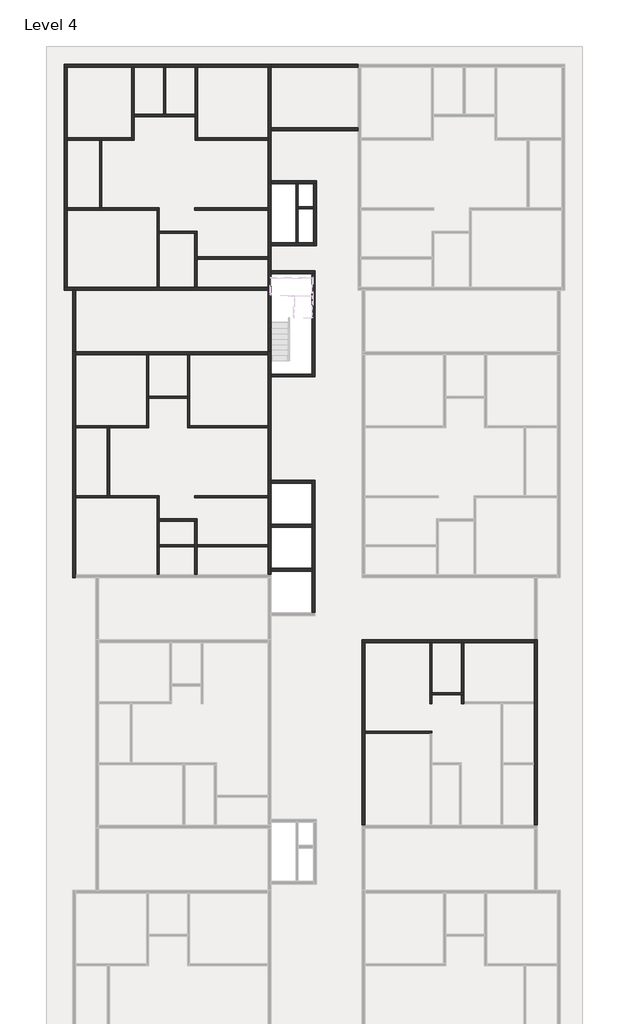
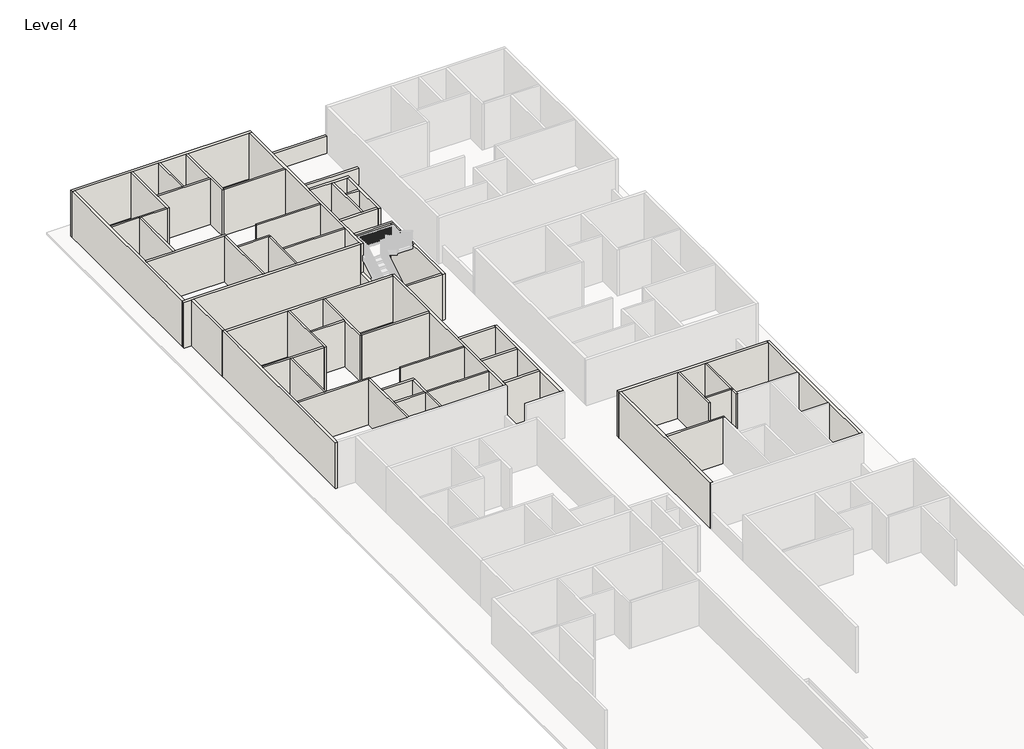
# One storey, part 3 of 8: 57 walls.
"""IFC4 building model written with IfcOpenShell, lengths in millimetres."""

from ifc_helpers import new_model, si_unit, frame, origin, place, context, project, spatial, polyline, outline, extrude, faceted_brep, element, save

model = new_model("IFC4")

# Units and contexts
model_context = context("Model", 3, world=origin())
ifc_project = project(units=[si_unit("LENGTHUNIT", "METRE", prefix="MILLI")], contexts=[model_context])

# Site, building, storey
site = spatial("IfcSite", under=ifc_project)
building = spatial("IfcBuilding", under=site)
storey = spatial("IfcBuildingStorey", under=building, Name="Level 4", Elevation=34378.6172466)

# Walls
placement = place(None, origin())
element("IfcWall", 1, ObjectType="4.5\"", at=placement, inside=storey, context=model_context, shape_type="Brep", body=[
    faceted_brep([(-10818.3415084, 35031.1216096, 34378.6172466), (-10818.3415084, 31373.5216096, 34378.6172466), (-10818.3415084, 31259.2216096, 34378.6172466), (-10818.3415084, 31259.2216096, 37426.6172466), (-10818.3415084, 31373.5216096, 37426.6172466), (-10818.3415084, 35031.1216096, 37426.6172466), (-10704.0415084, 35031.1216096, 34378.6172466), (-10704.0415084, 35031.1216096, 37426.6172466), (-10704.0415084, 32592.7216096, 37426.6172466), (-10704.0415084, 32478.4216096, 37426.6172466), (-10704.0415084, 31259.2216096, 37426.6172466), (-10704.0415084, 31259.2216096, 34378.6172466), (-10704.0415084, 32478.4216096, 34378.6172466), (-10704.0415084, 32592.7216096, 34378.6172466)], [[[0, 1, 2, 3, 4, 5]], [[6, 7, 8, 9, 10, 11, 12, 13]], [[2, 1, 0, 6, 13, 12, 11]], [[0, 5, 7, 6]], [[3, 2, 11, 10]], [[5, 4, 3, 10, 9, 8, 7]]]),
])
element("IfcWall", 2, ObjectType="4.5\"", at=placement, inside=storey, context=model_context, shape_type="Brep", body=[
    faceted_brep([(-10818.3415084, 31373.5216096, 34378.6172466), (-14171.1415084, 31373.5216096, 34378.6172466), (-14171.1415084, 31373.5216096, 37426.6172466), (-10818.3415084, 31373.5216096, 37426.6172466), (-10818.3415084, 31259.2216096, 34378.6172466), (-10818.3415084, 31259.2216096, 37426.6172466), (-12380.4415084, 31259.2216096, 37426.6172466), (-12494.7415084, 31259.2216096, 37426.6172466), (-14171.1415084, 31259.2216096, 37426.6172466), (-14171.1415084, 31259.2216096, 34378.6172466), (-12494.7415084, 31259.2216096, 34378.6172466), (-12380.4415084, 31259.2216096, 34378.6172466)], [[[0, 1, 2, 3]], [[4, 5, 6, 7, 8, 9, 10, 11]], [[1, 0, 4, 11, 10, 9]], [[0, 3, 5, 4]], [[2, 1, 9, 8]], [[3, 2, 8, 7, 6, 5]]]),
])
element("IfcWall", 3, ObjectType="4.5\"", at=placement, inside=storey, context=model_context, shape_type="SweptSolid", body=[
    extrude(outline(polyline([(-12494.7415084, 27754.0216096), (-12494.7415084, 31259.2216096), (-12380.4415084, 31259.2216096), (-12380.4415084, 27754.0216096), (-12494.7415084, 27754.0216096)])), frame((0.0, 0.0, 34378.6172466), z_axis=(0.0, 0.0, 1.0), x_axis=(1.0, 0.0, 0.0)), (0.0, 0.0, 1.0), 3048.0),
])
element("IfcWall", 4, ObjectType="4.5\"", at=placement, inside=storey, context=model_context, shape_type="Brep", body=[
    faceted_brep([(-14171.1415084, 27639.7216096, 34378.6172466), (-9510.2415084, 27639.7216096, 34378.6172466), (-9395.9415084, 27639.7216096, 34378.6172466), (-9395.9415084, 27639.7216096, 37426.6172466), (-9510.2415084, 27639.7216096, 37426.6172466), (-14171.1415084, 27639.7216096, 37426.6172466), (-14171.1415084, 27754.0216096, 34378.6172466), (-14171.1415084, 27754.0216096, 37426.6172466), (-12494.7415084, 27754.0216096, 37426.6172466), (-12380.4415084, 27754.0216096, 37426.6172466), (-9395.9415084, 27754.0216096, 37426.6172466), (-9395.9415084, 27754.0216096, 34378.6172466), (-12380.4415084, 27754.0216096, 34378.6172466), (-12494.7415084, 27754.0216096, 34378.6172466)], [[[0, 1, 2, 3, 4, 5]], [[6, 7, 8, 9, 10, 11, 12, 13]], [[2, 1, 0, 6, 13, 12, 11]], [[0, 5, 7, 6]], [[3, 2, 11, 10]], [[5, 4, 3, 10, 9, 8, 7]]]),
])
element("IfcWall", 5, ObjectType="4.5\"", at=placement, inside=storey, context=model_context, shape_type="Brep", body=[
    faceted_brep([(-9510.2415084, 27639.7216096, 34378.6172466), (-9510.2415084, 23651.9216096, 34378.6172466), (-9510.2415084, 23651.9216096, 37426.6172466), (-9510.2415084, 27639.7216096, 37426.6172466), (-9395.9415084, 27639.7216096, 34378.6172466), (-9395.9415084, 27639.7216096, 37426.6172466), (-9395.9415084, 26547.5216096, 37426.6172466), (-9395.9415084, 26433.2216096, 37426.6172466), (-9395.9415084, 23651.9216096, 37426.6172466), (-9395.9415084, 23651.9216096, 34378.6172466), (-9395.9415084, 26433.2216096, 34378.6172466), (-9395.9415084, 26547.5216096, 34378.6172466)], [[[0, 1, 2, 3]], [[4, 5, 6, 7, 8, 9, 10, 11]], [[1, 0, 4, 11, 10, 9]], [[0, 3, 5, 4]], [[2, 1, 9, 8]], [[3, 2, 8, 7, 6, 5]]]),
])
element("IfcWall", 6, ObjectType="4.5\"", at=placement, inside=storey, context=model_context, shape_type="Brep", body=[
    faceted_brep([(-9395.9415084, 26433.2216096, 34378.6172466), (-7567.1415084, 26433.2216096, 34378.6172466), (-7452.8415084, 26433.2216096, 34378.6172466), (-7452.8415084, 26433.2216096, 37426.6172466), (-7567.1415084, 26433.2216096, 37426.6172466), (-9395.9415084, 26433.2216096, 37426.6172466), (-9395.9415084, 26547.5216096, 34378.6172466), (-9395.9415084, 26547.5216096, 37426.6172466), (-7452.8415084, 26547.5216096, 37426.6172466), (-7452.8415084, 26547.5216096, 34378.6172466)], [[[0, 1, 2, 3, 4, 5]], [[6, 7, 8, 9]], [[2, 1, 0, 6, 9]], [[0, 5, 7, 6]], [[3, 2, 9, 8]], [[5, 4, 3, 8, 7]]]),
])
element("IfcWall", 7, ObjectType="4.5\"", at=placement, inside=storey, context=model_context, shape_type="Brep", body=[
    faceted_brep([(-7567.1415084, 26433.2216096, 34378.6172466), (-7567.1415084, 23651.9216096, 34378.6172466), (-7567.1415084, 23651.9216096, 37426.6172466), (-7567.1415084, 26433.2216096, 37426.6172466), (-7452.8415084, 26433.2216096, 34378.6172466), (-7452.8415084, 26433.2216096, 37426.6172466), (-7452.8415084, 25214.0216096, 37426.6172466), (-7452.8415084, 25099.7216096, 37426.6172466), (-7452.8415084, 23651.9216096, 37426.6172466), (-7452.8415084, 23651.9216096, 34378.6172466), (-7452.8415084, 25099.7216096, 34378.6172466), (-7452.8415084, 25214.0216096, 34378.6172466)], [[[0, 1, 2, 3]], [[4, 5, 6, 7, 8, 9, 10, 11]], [[1, 0, 4, 11, 10, 9]], [[0, 3, 5, 4]], [[2, 1, 9, 8]], [[3, 2, 8, 7, 6, 5]]]),
])
element("IfcWall", 8, ObjectType="4.5\"", at=placement, inside=storey, context=model_context, shape_type="SweptSolid", body=[
    extrude(outline(polyline([(-7452.8415084, 25214.0216096), (-3769.8415084, 25214.0216096), (-3769.8415084, 25099.7216096), (-7452.8415084, 25099.7216096), (-7452.8415084, 25214.0216096)])), frame((0.0, 0.0, 34378.6172466), z_axis=(0.0, 0.0, 1.0), x_axis=(1.0, 0.0, 0.0)), (0.0, 0.0, 1.0), 3048.0),
])
element("IfcWall", 9, ObjectType="4.5\"", at=placement, inside=storey, context=model_context, shape_type="SweptSolid", body=[
    extrude(outline(polyline([(-3769.8415084, 27639.7216096), (-7567.1415084, 27639.7216096), (-7567.1415084, 27754.0216096), (-3769.8415084, 27754.0216096), (-3769.8415084, 27639.7216096)])), frame((0.0, 0.0, 34378.6172466), z_axis=(0.0, 0.0, 1.0), x_axis=(1.0, 0.0, 0.0)), (0.0, 0.0, 1.0), 3048.0),
])
element("IfcWall", 10, ObjectType="4.5\"", at=placement, inside=storey, context=model_context, shape_type="Brep", body=[
    faceted_brep([(-10704.0415084, 32478.4216096, 34378.6172466), (-7541.7415084, 32478.4216096, 34378.6172466), (-7541.7415084, 32478.4216096, 37426.6172466), (-10704.0415084, 32478.4216096, 37426.6172466), (-10704.0415084, 32592.7216096, 34378.6172466), (-10704.0415084, 32592.7216096, 37426.6172466), (-9180.0415084, 32592.7216096, 37426.6172466), (-9065.7415084, 32592.7216096, 37426.6172466), (-7541.7415084, 32592.7216096, 37426.6172466), (-7541.7415084, 32592.7216096, 34378.6172466), (-9065.7415084, 32592.7216096, 34378.6172466), (-9180.0415084, 32592.7216096, 34378.6172466)], [[[0, 1, 2, 3]], [[4, 5, 6, 7, 8, 9, 10, 11]], [[1, 0, 4, 11, 10, 9]], [[0, 3, 5, 4]], [[2, 1, 9, 8]], [[3, 2, 8, 7, 6, 5]]]),
])
element("IfcWall", 11, ObjectType="4.5\"", at=placement, inside=storey, context=model_context, shape_type="SweptSolid", body=[
    extrude(outline(polyline([(-9180.0415084, 32592.7216096), (-9180.0415084, 35031.1216096), (-9065.7415084, 35031.1216096), (-9065.7415084, 32592.7216096), (-9180.0415084, 32592.7216096)])), frame((0.0, 0.0, 34378.6172466), z_axis=(0.0, 0.0, 1.0), x_axis=(1.0, 0.0, 0.0)), (0.0, 0.0, 1.0), 3048.0),
])
element("IfcWall", 12, ObjectType="4.5\"", at=placement, inside=storey, context=model_context, shape_type="Brep", body=[
    faceted_brep([(-7541.7415084, 35031.1216096, 34378.6172466), (-7541.7415084, 32592.7216096, 34378.6172466), (-7541.7415084, 32478.4216096, 34378.6172466), (-7541.7415084, 31259.2216096, 34378.6172466), (-7541.7415084, 31259.2216096, 37426.6172466), (-7541.7415084, 32478.4216096, 37426.6172466), (-7541.7415084, 32592.7216096, 37426.6172466), (-7541.7415084, 35031.1216096, 37426.6172466), (-7427.4415084, 35031.1216096, 34378.6172466), (-7427.4415084, 35031.1216096, 37426.6172466), (-7427.4415084, 31373.5216096, 37426.6172466), (-7427.4415084, 31259.2216096, 37426.6172466), (-7427.4415084, 31259.2216096, 34378.6172466), (-7427.4415084, 31373.5216096, 34378.6172466)], [[[0, 1, 2, 3, 4, 5, 6, 7]], [[8, 9, 10, 11, 12, 13]], [[3, 2, 1, 0, 8, 13, 12]], [[0, 7, 9, 8]], [[4, 3, 12, 11]], [[7, 6, 5, 4, 11, 10, 9]]]),
])
element("IfcWall", 13, ObjectType="4.5\"", at=placement, inside=storey, context=model_context, shape_type="SweptSolid", body=[
    extrude(outline(polyline([(-3769.8415084, 31259.2216096), (-7427.4415084, 31259.2216096), (-7427.4415084, 31373.5216096), (-3769.8415084, 31373.5216096), (-3769.8415084, 31259.2216096)])), frame((0.0, 0.0, 34378.6172466), z_axis=(0.0, 0.0, 1.0), x_axis=(1.0, 0.0, 0.0)), (0.0, 0.0, 1.0), 3048.0),
])
element("IfcWall", 14, ObjectType="4.5\"", at=placement, inside=storey, context=model_context, shape_type="Brep", body=[
    faceted_brep([(-10061.4044854, 20146.7216096, 34378.6172466), (-10061.4044854, 16489.1216096, 34378.6172466), (-10061.4044854, 16374.8216096, 34378.6172466), (-10061.4044854, 16374.8216096, 37426.6172466), (-10061.4044854, 16489.1216096, 37426.6172466), (-10061.4044854, 20146.7216096, 37426.6172466), (-9947.1044854, 20146.7216096, 34378.6172466), (-9947.1044854, 20146.7216096, 37426.6172466), (-9947.1044854, 18013.1216096, 37426.6172466), (-9947.1044854, 17898.8216096, 37426.6172466), (-9947.1044854, 16374.8216096, 37426.6172466), (-9947.1044854, 16374.8216096, 34378.6172466), (-9947.1044854, 17898.8216096, 34378.6172466), (-9947.1044854, 18013.1216096, 34378.6172466)], [[[0, 1, 2, 3, 4, 5]], [[6, 7, 8, 9, 10, 11, 12, 13]], [[2, 1, 0, 6, 13, 12, 11]], [[0, 5, 7, 6]], [[3, 2, 11, 10]], [[5, 4, 3, 10, 9, 8, 7]]]),
])
element("IfcWall", 15, ObjectType="4.5\"", at=placement, inside=storey, context=model_context, shape_type="Brep", body=[
    faceted_brep([(-10061.4044854, 16489.1216096, 34378.6172466), (-13719.0044854, 16489.1216096, 34378.6172466), (-13719.0044854, 16489.1216096, 37426.6172466), (-10061.4044854, 16489.1216096, 37426.6172466), (-10061.4044854, 16374.8216096, 34378.6172466), (-10061.4044854, 16374.8216096, 37426.6172466), (-11980.3915084, 16374.8216096, 37426.6172466), (-12094.6915084, 16374.8216096, 37426.6172466), (-13719.0044854, 16374.8216096, 37426.6172466), (-13719.0044854, 16374.8216096, 34378.6172466), (-12094.6915084, 16374.8216096, 34378.6172466), (-11980.3915084, 16374.8216096, 34378.6172466)], [[[0, 1, 2, 3]], [[4, 5, 6, 7, 8, 9, 10, 11]], [[1, 0, 4, 11, 10, 9]], [[0, 3, 5, 4]], [[2, 1, 9, 8]], [[3, 2, 8, 7, 6, 5]]]),
])
element("IfcWall", 16, ObjectType="4.5\"", at=placement, inside=storey, context=model_context, shape_type="SweptSolid", body=[
    extrude(outline(polyline([(-7940.5044854, 17898.8216096), (-9947.1044854, 17898.8216096), (-9947.1044854, 18013.1216096), (-7940.5044854, 18013.1216096), (-7940.5044854, 17898.8216096)])), frame((0.0, 0.0, 34378.6172466), z_axis=(0.0, 0.0, 1.0), x_axis=(1.0, 0.0, 0.0)), (0.0, 0.0, 1.0), 3048.0),
])
element("IfcWall", 17, ObjectType="4.5\"", at=placement, inside=storey, context=model_context, shape_type="Brep", body=[
    faceted_brep([(-7940.5044854, 20146.7216096, 34378.6172466), (-7940.5044854, 18013.1216096, 34378.6172466), (-7940.5044854, 17898.8216096, 34378.6172466), (-7940.5044854, 16374.8216096, 34378.6172466), (-7940.5044854, 16374.8216096, 37426.6172466), (-7940.5044854, 17898.8216096, 37426.6172466), (-7940.5044854, 18013.1216096, 37426.6172466), (-7940.5044854, 20146.7216096, 37426.6172466), (-7826.2044854, 20146.7216096, 34378.6172466), (-7826.2044854, 20146.7216096, 37426.6172466), (-7826.2044854, 16489.1216096, 37426.6172466), (-7826.2044854, 16374.8216096, 37426.6172466), (-7826.2044854, 16374.8216096, 34378.6172466), (-7826.2044854, 16489.1216096, 34378.6172466)], [[[0, 1, 2, 3, 4, 5, 6, 7]], [[8, 9, 10, 11, 12, 13]], [[3, 2, 1, 0, 8, 13, 12]], [[0, 7, 9, 8]], [[4, 3, 12, 11]], [[7, 6, 5, 4, 11, 10, 9]]]),
])
element("IfcWall", 18, ObjectType="4.5\"", at=placement, inside=storey, context=model_context, shape_type="SweptSolid", body=[
    extrude(outline(polyline([(-3769.8415084, 16374.8216096), (-7826.2044854, 16374.8216096), (-7826.2044854, 16489.1216096), (-3769.8415084, 16489.1216096), (-3769.8415084, 16374.8216096)])), frame((0.0, 0.0, 34378.6172466), z_axis=(0.0, 0.0, 1.0), x_axis=(1.0, 0.0, 0.0)), (0.0, 0.0, 1.0), 3048.0),
])
element("IfcWall", 19, ObjectType="4.5\"", at=placement, inside=storey, context=model_context, shape_type="SweptSolid", body=[
    extrude(outline(polyline([(-12094.6915084, 12869.6216096), (-12094.6915084, 16374.8216096), (-11980.3915084, 16374.8216096), (-11980.3915084, 12869.6216096), (-12094.6915084, 12869.6216096)])), frame((0.0, 0.0, 34378.6172466), z_axis=(0.0, 0.0, 1.0), x_axis=(1.0, 0.0, 0.0)), (0.0, 0.0, 1.0), 3048.0),
])
element("IfcWall", 20, ObjectType="4.5\"", at=placement, inside=storey, context=model_context, shape_type="Brep", body=[
    faceted_brep([(-13719.0044854, 12755.3216096, 34378.6172466), (-9510.2415084, 12755.3216096, 34378.6172466), (-9395.9415084, 12755.3216096, 34378.6172466), (-9395.9415084, 12755.3216096, 37426.6172466), (-9510.2415084, 12755.3216096, 37426.6172466), (-13719.0044854, 12755.3216096, 37426.6172466), (-13719.0044854, 12869.6216096, 34378.6172466), (-13719.0044854, 12869.6216096, 37426.6172466), (-12094.6915084, 12869.6216096, 37426.6172466), (-11980.3915084, 12869.6216096, 37426.6172466), (-9395.9415084, 12869.6216096, 37426.6172466), (-9395.9415084, 12869.6216096, 34378.6172466), (-11980.3915084, 12869.6216096, 34378.6172466), (-12094.6915084, 12869.6216096, 34378.6172466)], [[[0, 1, 2, 3, 4, 5]], [[6, 7, 8, 9, 10, 11, 12, 13]], [[2, 1, 0, 6, 13, 12, 11]], [[0, 5, 7, 6]], [[3, 2, 11, 10]], [[5, 4, 3, 10, 9, 8, 7]]]),
])
element("IfcWall", 21, ObjectType="4.5\"", at=placement, inside=storey, context=model_context, shape_type="Brep", body=[
    faceted_brep([(-9510.2415084, 12755.3216096, 34378.6172466), (-9510.2415084, 8767.5216096, 34378.6172466), (-9510.2415084, 8767.5216096, 37426.6172466), (-9510.2415084, 12755.3216096, 37426.6172466), (-9395.9415084, 12755.3216096, 34378.6172466), (-9395.9415084, 12755.3216096, 37426.6172466), (-9395.9415084, 11663.1216096, 37426.6172466), (-9395.9415084, 11548.8216096, 37426.6172466), (-9395.9415084, 10329.6216096, 37426.6172466), (-9395.9415084, 10215.3216096, 37426.6172466), (-9395.9415084, 8767.5216096, 37426.6172466), (-9395.9415084, 8767.5216096, 34378.6172466), (-9395.9415084, 10215.3216096, 34378.6172466), (-9395.9415084, 10329.6216096, 34378.6172466), (-9395.9415084, 11548.8216096, 34378.6172466), (-9395.9415084, 11663.1216096, 34378.6172466)], [[[0, 1, 2, 3]], [[4, 5, 6, 7, 8, 9, 10, 11, 12, 13, 14, 15]], [[1, 0, 4, 15, 14, 13, 12, 11]], [[0, 3, 5, 4]], [[2, 1, 11, 10]], [[3, 2, 10, 9, 8, 7, 6, 5]]]),
])
element("IfcWall", 22, ObjectType="4.5\"", at=placement, inside=storey, context=model_context, shape_type="SweptSolid", body=[
    extrude(outline(polyline([(-7567.1415084, 10215.3216096), (-9395.9415084, 10215.3216096), (-9395.9415084, 10329.6216096), (-7567.1415084, 10329.6216096), (-7567.1415084, 10215.3216096)])), frame((0.0, 0.0, 34378.6172466), z_axis=(0.0, 0.0, 1.0), x_axis=(1.0, 0.0, 0.0)), (0.0, 0.0, 1.0), 3048.0),
])
element("IfcWall", 23, ObjectType="4.5\"", at=placement, inside=storey, context=model_context, shape_type="Brep", body=[
    faceted_brep([(-9395.9415084, 11548.8216096, 34378.6172466), (-7567.1415084, 11548.8216096, 34378.6172466), (-7452.8415084, 11548.8216096, 34378.6172466), (-7452.8415084, 11548.8216096, 37426.6172466), (-7567.1415084, 11548.8216096, 37426.6172466), (-9395.9415084, 11548.8216096, 37426.6172466), (-9395.9415084, 11663.1216096, 34378.6172466), (-9395.9415084, 11663.1216096, 37426.6172466), (-7452.8415084, 11663.1216096, 37426.6172466), (-7452.8415084, 11663.1216096, 34378.6172466)], [[[0, 1, 2, 3, 4, 5]], [[6, 7, 8, 9]], [[2, 1, 0, 6, 9]], [[0, 5, 7, 6]], [[3, 2, 9, 8]], [[5, 4, 3, 8, 7]]]),
])
element("IfcWall", 24, ObjectType="4.5\"", at=placement, inside=storey, context=model_context, shape_type="Brep", body=[
    faceted_brep([(-7567.1415084, 11548.8216096, 34378.6172466), (-7567.1415084, 10329.6216096, 34378.6172466), (-7567.1415084, 10215.3216096, 34378.6172466), (-7567.1415084, 8767.5216096, 34378.6172466), (-7567.1415084, 8767.5216096, 37426.6172466), (-7567.1415084, 10215.3216096, 37426.6172466), (-7567.1415084, 10329.6216096, 37426.6172466), (-7567.1415084, 11548.8216096, 37426.6172466), (-7452.8415084, 11548.8216096, 34378.6172466), (-7452.8415084, 11548.8216096, 37426.6172466), (-7452.8415084, 10329.6216096, 37426.6172466), (-7452.8415084, 10215.3216096, 37426.6172466), (-7452.8415084, 8767.5216096, 37426.6172466), (-7452.8415084, 8767.5216096, 34378.6172466), (-7452.8415084, 10215.3216096, 34378.6172466), (-7452.8415084, 10329.6216096, 34378.6172466)], [[[0, 1, 2, 3, 4, 5, 6, 7]], [[8, 9, 10, 11, 12, 13, 14, 15]], [[3, 2, 1, 0, 8, 15, 14, 13]], [[0, 7, 9, 8]], [[4, 3, 13, 12]], [[7, 6, 5, 4, 12, 11, 10, 9]]]),
])
element("IfcWall", 25, ObjectType="4.5\"", at=placement, inside=storey, context=model_context, shape_type="SweptSolid", body=[
    extrude(outline(polyline([(-3769.8415084, 10215.3216096), (-7452.8415084, 10215.3216096), (-7452.8415084, 10329.6216096), (-3769.8415084, 10329.6216096), (-3769.8415084, 10215.3216096)])), frame((0.0, 0.0, 34378.6172466), z_axis=(0.0, 0.0, 1.0), x_axis=(1.0, 0.0, 0.0)), (0.0, 0.0, 1.0), 3048.0),
])
element("IfcWall", 26, ObjectType="4.5\"", at=placement, inside=storey, context=model_context, shape_type="SweptSolid", body=[
    extrude(outline(polyline([(-3769.8415084, 12755.3216096), (-7567.1415084, 12755.3216096), (-7567.1415084, 12869.6216096), (-3769.8415084, 12869.6216096), (-3769.8415084, 12755.3216096)])), frame((0.0, 0.0, 34378.6172466), z_axis=(0.0, 0.0, 1.0), x_axis=(1.0, 0.0, 0.0)), (0.0, 0.0, 1.0), 3048.0),
])
element("IfcWall", 27, ObjectType="4.5\"", at=placement, inside=storey, context=model_context, shape_type="Brep", body=[
    faceted_brep([(1259.3584916, 572.7745083, 34378.6172466), (4610.8714687, 572.7745083, 34378.6172466), (4725.1714687, 572.7745083, 34378.6172466), (4725.1714687, 572.7745083, 37426.6172466), (4610.8714687, 572.7745083, 37426.6172466), (1259.3584916, 572.7745083, 37426.6172466), (1259.3584916, 687.0745083, 34378.6172466), (1259.3584916, 687.0745083, 37426.6172466), (4725.1714687, 687.0745083, 37426.6172466), (4725.1714687, 687.0745083, 34378.6172466)], [[[0, 1, 2, 3, 4, 5]], [[6, 7, 8, 9]], [[2, 1, 0, 6, 9]], [[0, 5, 7, 6]], [[3, 2, 9, 8]], [[5, 4, 3, 8, 7]]]),
])
element("IfcWall", 28, ObjectType="4.5\"", at=placement, inside=storey, context=model_context, shape_type="Brep", body=[
    faceted_brep([(4610.8714687, 5262.3216096, 34378.6172466), (4610.8714687, 2100.0216096, 34378.6172466), (4610.8714687, 2100.0216096, 37426.6172466), (4610.8714687, 5262.3216096, 37426.6172466), (4725.1714687, 5262.3216096, 34378.6172466), (4725.1714687, 5262.3216096, 37426.6172466), (4725.1714687, 2671.5216096, 37426.6172466), (4725.1714687, 2557.2216096, 37426.6172466), (4725.1714687, 2100.0216096, 37426.6172466), (4725.1714687, 2100.0216096, 34378.6172466), (4725.1714687, 2557.2216096, 34378.6172466), (4725.1714687, 2671.5216096, 34378.6172466)], [[[0, 1, 2, 3]], [[4, 5, 6, 7, 8, 9, 10, 11]], [[1, 0, 4, 11, 10, 9]], [[2, 1, 9, 8]], [[0, 3, 5, 4]], [[3, 2, 8, 7, 6, 5]]]),
])
element("IfcWall", 29, ObjectType="4.5\"", at=placement, inside=storey, context=model_context, shape_type="Brep", body=[
    faceted_brep([(4725.1714687, 2557.2216096, 34378.6172466), (6249.1714687, 2557.2216096, 34378.6172466), (6363.4714687, 2557.2216096, 34378.6172466), (6363.4714687, 2557.2216096, 37426.6172466), (6249.1714687, 2557.2216096, 37426.6172466), (4725.1714687, 2557.2216096, 37426.6172466), (4725.1714687, 2671.5216096, 34378.6172466), (4725.1714687, 2671.5216096, 37426.6172466), (6249.1714687, 2671.5216096, 37426.6172466), (6363.4714687, 2671.5216096, 37426.6172466), (6363.4714687, 2671.5216096, 34378.6172466), (6249.1714687, 2671.5216096, 34378.6172466)], [[[0, 1, 2, 3, 4, 5]], [[6, 7, 8, 9, 10, 11]], [[2, 1, 0, 6, 11, 10]], [[0, 5, 7, 6]], [[3, 2, 10, 9]], [[5, 4, 3, 9, 8, 7]]]),
])
element("IfcWall", 30, ObjectType="4.5\"", at=placement, inside=storey, context=model_context, shape_type="SweptSolid", body=[
    extrude(outline(polyline([(6363.4714687, 5262.3216096), (6363.4714687, 2671.5216096), (6249.1714687, 2671.5216096), (6249.1714687, 5262.3216096), (6363.4714687, 5262.3216096)])), frame((0.0, 0.0, 34378.6172466), z_axis=(0.0, 0.0, 1.0), x_axis=(1.0, 0.0, 0.0)), (0.0, 0.0, 1.0), 3048.0),
])
element("IfcWall", 31, ObjectType="4.5\"", at=placement, inside=storey, context=model_context, shape_type="Brep", body=[
    faceted_brep([(6249.1714687, 2557.2216096, 34378.6172466), (6249.1714687, 2100.0216096, 34378.6172466), (6249.1714687, 2100.0216096, 37426.6172466), (6249.1714687, 2557.2216096, 37426.6172466), (6363.4714687, 2557.2216096, 34378.6172466), (6363.4714687, 2557.2216096, 37426.6172466), (6363.4714687, 2214.3216096, 37426.6172466), (6363.4714687, 2100.0216096, 37426.6172466), (6363.4714687, 2100.0216096, 34378.6172466), (6363.4714687, 2214.3216096, 34378.6172466)], [[[0, 1, 2, 3]], [[4, 5, 6, 7, 8, 9]], [[1, 0, 4, 9, 8]], [[0, 3, 5, 4]], [[2, 1, 8, 7]], [[3, 2, 7, 6, 5]]]),
])
element("IfcWall", 32, ObjectType="4.5\"", at=placement, inside=storey, context=model_context, shape_type="Brep", body=[
    faceted_brep([(-2321.9738684, 29000.0900967, 34378.6172466), (-2321.9738684, 25952.0900967, 34378.6172466), (-2321.9738684, 25952.0900967, 37426.6172466), (-2321.9738684, 29000.0900967, 37426.6172466), (-2207.6738684, 29000.0900967, 34378.6172466), (-2207.6738684, 29000.0900967, 37426.6172466), (-2207.6738684, 27820.8172885, 37426.6172466), (-2207.6738684, 27706.5172885, 37426.6172466), (-2207.6738684, 25952.0900967, 37426.6172466), (-2207.6738684, 25952.0900967, 34378.6172466), (-2207.6738684, 27706.5172885, 34378.6172466), (-2207.6738684, 27820.8172885, 34378.6172466)], [[[0, 1, 2, 3]], [[4, 5, 6, 7, 8, 9, 10, 11]], [[1, 0, 4, 11, 10, 9]], [[3, 2, 8, 7, 6, 5]], [[0, 3, 5, 4]], [[2, 1, 9, 8]]]),
])
element("IfcWall", 33, ObjectType="4.5\"", at=placement, inside=storey, context=model_context, shape_type="SweptSolid", body=[
    extrude(outline(polyline([(-2207.6738684, 27820.8172885), (-1407.6415084, 27820.8172885), (-1407.6415084, 27706.5172885), (-2207.6738684, 27706.5172885), (-2207.6738684, 27820.8172885)])), frame((0.0, 0.0, 34378.6172466), z_axis=(0.0, 0.0, 1.0), x_axis=(1.0, 0.0, 0.0)), (0.0, 0.0, 1.0), 3048.0),
])
element("IfcWall", 34, ObjectType="6\"", at=placement, inside=storey, context=model_context, shape_type="Brep", body=[
    faceted_brep([(-14323.5415084, 35031.1216096, 34378.6172466), (-14171.1415084, 35031.1216096, 34378.6172466), (-10818.3415084, 35031.1216096, 34378.6172466), (-10704.0415084, 35031.1216096, 34378.6172466), (-9180.0415084, 35031.1216096, 34378.6172466), (-9065.7415084, 35031.1216096, 34378.6172466), (-7541.7415084, 35031.1216096, 34378.6172466), (-7427.4415084, 35031.1216096, 34378.6172466), (-3769.8415084, 35031.1216096, 34378.6172466), (-3617.4415084, 35031.1216096, 34378.6172466), (-3617.4415084, 35031.1216096, 37426.6172466), (-3769.8415084, 35031.1216096, 37426.6172466), (-7427.4415084, 35031.1216096, 37426.6172466), (-7541.7415084, 35031.1216096, 37426.6172466), (-9065.7415084, 35031.1216096, 37426.6172466), (-9180.0415084, 35031.1216096, 37426.6172466), (-10704.0415084, 35031.1216096, 37426.6172466), (-10818.3415084, 35031.1216096, 37426.6172466), (-14171.1415084, 35031.1216096, 37426.6172466), (-14323.5415084, 35031.1216096, 37426.6172466), (-14323.5415084, 35183.5216096, 34378.6172466), (-14323.5415084, 35183.5216096, 37426.6172466), (-3617.4415084, 35183.5216096, 37426.6172466), (-3617.4415084, 35183.5216096, 34378.6172466)], [[[0, 1, 2, 3, 4, 5, 6, 7, 8, 9, 10, 11, 12, 13, 14, 15, 16, 17, 18, 19]], [[20, 21, 22, 23]], [[9, 8, 7, 6, 5, 4, 3, 2, 1, 0, 20, 23]], [[0, 19, 21, 20]], [[9, 23, 22, 10]], [[19, 18, 17, 16, 15, 14, 13, 12, 11, 10, 22, 21]]]),
])
element("IfcWall", 35, ObjectType="6\"", at=placement, inside=storey, context=model_context, shape_type="Brep", body=[
    faceted_brep([(-3769.8415084, 35031.1216096, 37426.6172466), (-3769.8415084, 35031.1216096, 34378.6172466), (-3769.8415084, 31373.5216096, 34378.6172466), (-3769.8415084, 31259.2216096, 34378.6172466), (-3769.8415084, 27754.0216096, 34378.6172466), (-3769.8415084, 27639.7216096, 34378.6172466), (-3769.8415084, 25214.0216096, 34378.6172466), (-3769.8415084, 25099.7216096, 34378.6172466), (-3769.8415084, 23651.9216096, 34378.6172466), (-3769.8415084, 23499.5216096, 34378.6172466), (-3769.8415084, 23499.5216096, 37426.6172466), (-3769.8415084, 23651.9216096, 37426.6172466), (-3769.8415084, 25099.7216096, 37426.6172466), (-3769.8415084, 25214.0216096, 37426.6172466), (-3769.8415084, 27639.7216096, 37426.6172466), (-3769.8415084, 27754.0216096, 37426.6172466), (-3769.8415084, 31259.2216096, 37426.6172466), (-3769.8415084, 31373.5216096, 37426.6172466), (-3617.4415084, 35031.1216096, 34378.6172466), (-3617.4415084, 35031.1216096, 37426.6172466), (-3617.4415084, 29152.4900967, 37426.6172466), (-3617.4415084, 29000.0900967, 37426.6172466), (-3617.4415084, 25952.0900967, 37426.6172466), (-3617.4415084, 25799.6900967, 37426.6172466), (-3617.4415084, 24490.1216096, 37426.6172466), (-3617.4415084, 24337.7216096, 37426.6172466), (-3617.4415084, 23499.5216096, 37426.6172466), (-3617.4415084, 23499.5216096, 34378.6172466), (-3617.4415084, 24337.7216096, 34378.6172466), (-3617.4415084, 24490.1216096, 34378.6172466), (-3617.4415084, 25799.6900967, 34378.6172466), (-3617.4415084, 25952.0900967, 34378.6172466), (-3617.4415084, 29000.0900967, 34378.6172466), (-3617.4415084, 29152.4900967, 34378.6172466), (-3617.4415084, 31744.9197155, 34378.6172466), (-3617.4415084, 31897.3197155, 34378.6172466)], [[[0, 1, 2, 3, 4, 5, 6, 7, 8, 9, 10, 11, 12, 13, 14, 15, 16, 17]], [[18, 19, 20, 21, 22, 23, 24, 25, 26, 27, 28, 29, 30, 31, 32, 33, 34, 35]], [[9, 8, 7, 6, 5, 4, 3, 2, 1, 18, 35, 34, 33, 32, 31, 30, 29, 28, 27]], [[0, 19, 18, 1]], [[9, 27, 26, 10]], [[0, 17, 16, 15, 14, 13, 12, 11, 10, 26, 25, 24, 23, 22, 21, 20, 19]]]),
])
element("IfcWall", 36, ObjectType="6\"", at=placement, inside=storey, context=model_context, shape_type="Brep", body=[
    faceted_brep([(-3769.8415084, 23651.9216096, 37426.6172466), (-3769.8415084, 23651.9216096, 34378.6172466), (-7452.8415084, 23651.9216096, 34378.6172466), (-7567.1415084, 23651.9216096, 34378.6172466), (-9395.9415084, 23651.9216096, 34378.6172466), (-9510.2415084, 23651.9216096, 34378.6172466), (-14171.1415084, 23651.9216096, 34378.6172466), (-14323.5415084, 23651.9216096, 34378.6172466), (-14323.5415084, 23651.9216096, 37426.6172466), (-14171.1415084, 23651.9216096, 37426.6172466), (-9510.2415084, 23651.9216096, 37426.6172466), (-9395.9415084, 23651.9216096, 37426.6172466), (-7567.1415084, 23651.9216096, 37426.6172466), (-7452.8415084, 23651.9216096, 37426.6172466), (-3769.8415084, 23499.5216096, 34378.6172466), (-3769.8415084, 23499.5216096, 37426.6172466), (-13719.0044854, 23499.5216096, 37426.6172466), (-13871.4044854, 23499.5216096, 37426.6172466), (-14323.5415084, 23499.5216096, 37426.6172466), (-14323.5415084, 23499.5216096, 34378.6172466), (-13871.4044854, 23499.5216096, 34378.6172466), (-13719.0044854, 23499.5216096, 34378.6172466)], [[[0, 1, 2, 3, 4, 5, 6, 7, 8, 9, 10, 11, 12, 13]], [[14, 15, 16, 17, 18, 19, 20, 21]], [[7, 6, 5, 4, 3, 2, 1, 14, 21, 20, 19]], [[8, 7, 19, 18]], [[0, 15, 14, 1]], [[0, 13, 12, 11, 10, 9, 8, 18, 17, 16, 15]]]),
])
element("IfcWall", 37, ObjectType="6\"", at=placement, inside=storey, context=model_context, shape_type="Brep", body=[
    faceted_brep([(-14171.1415084, 23651.9216096, 34378.6172466), (-14171.1415084, 27639.7216096, 34378.6172466), (-14171.1415084, 27754.0216096, 34378.6172466), (-14171.1415084, 31259.2216096, 34378.6172466), (-14171.1415084, 31373.5216096, 34378.6172466), (-14171.1415084, 35031.1216096, 34378.6172466), (-14171.1415084, 35031.1216096, 37426.6172466), (-14171.1415084, 31373.5216096, 37426.6172466), (-14171.1415084, 31259.2216096, 37426.6172466), (-14171.1415084, 27754.0216096, 37426.6172466), (-14171.1415084, 27639.7216096, 37426.6172466), (-14171.1415084, 23651.9216096, 37426.6172466), (-14323.5415084, 23651.9216096, 34378.6172466), (-14323.5415084, 23651.9216096, 37426.6172466), (-14323.5415084, 35031.1216096, 37426.6172466), (-14323.5415084, 35031.1216096, 34378.6172466)], [[[0, 1, 2, 3, 4, 5, 6, 7, 8, 9, 10, 11]], [[12, 13, 14, 15]], [[5, 4, 3, 2, 1, 0, 12, 15]], [[6, 5, 15, 14]], [[0, 11, 13, 12]], [[11, 10, 9, 8, 7, 6, 14, 13]]]),
])
element("IfcWall", 38, ObjectType="6\"", at=placement, inside=storey, context=model_context, shape_type="Brep", body=[
    faceted_brep([(-13871.4044854, 20299.1216096, 34378.6172466), (-13871.4044854, 8615.1216096, 34378.6172466), (-13871.4044854, 8615.1216096, 37426.6172466), (-13871.4044854, 20299.1216096, 37426.6172466), (-13719.0044854, 20299.1216096, 34378.6172466), (-13719.0044854, 20299.1216096, 37426.6172466), (-13719.0044854, 20146.7216096, 37426.6172466), (-13719.0044854, 16489.1216096, 37426.6172466), (-13719.0044854, 16374.8216096, 37426.6172466), (-13719.0044854, 12869.6216096, 37426.6172466), (-13719.0044854, 12755.3216096, 37426.6172466), (-13719.0044854, 8767.5216096, 37426.6172466), (-13719.0044854, 8615.1216096, 37426.6172466), (-13719.0044854, 8615.1216096, 34378.6172466), (-13719.0044854, 8767.5216096, 34378.6172466), (-13719.0044854, 12755.3216096, 34378.6172466), (-13719.0044854, 12869.6216096, 34378.6172466), (-13719.0044854, 16374.8216096, 34378.6172466), (-13719.0044854, 16489.1216096, 34378.6172466), (-13719.0044854, 20146.7216096, 34378.6172466)], [[[0, 1, 2, 3]], [[4, 5, 6, 7, 8, 9, 10, 11, 12, 13, 14, 15, 16, 17, 18, 19]], [[1, 0, 4, 19, 18, 17, 16, 15, 14, 13]], [[2, 1, 13, 12]], [[0, 3, 5, 4]], [[3, 2, 12, 11, 10, 9, 8, 7, 6, 5]]]),
])
element("IfcWall", 39, ObjectType="6\"", at=placement, inside=storey, context=model_context, shape_type="Brep", body=[
    faceted_brep([(-3617.4415084, 8767.5216096, 37426.6172466), (-3617.4415084, 8767.5216096, 34378.6172466), (-3617.4415084, 8945.2303368, 34378.6172466), (-3617.4415084, 9097.6303368, 34378.6172466), (-3617.4415084, 11231.2303368, 34378.6172466), (-3617.4415084, 11383.6303368, 34378.6172466), (-3617.4415084, 13517.2303368, 34378.6172466), (-3617.4415084, 13669.6303368, 34378.6172466), (-3617.4415084, 19003.7216096, 34378.6172466), (-3617.4415084, 19156.1216096, 34378.6172466), (-3617.4415084, 20299.1216096, 34378.6172466), (-3617.4415084, 20299.1216096, 37426.6172466), (-3617.4415084, 19156.1216096, 37426.6172466), (-3617.4415084, 19003.7216096, 37426.6172466), (-3617.4415084, 13669.6303368, 37426.6172466), (-3617.4415084, 13517.2303368, 37426.6172466), (-3617.4415084, 11383.6303368, 37426.6172466), (-3617.4415084, 11231.2303368, 37426.6172466), (-3617.4415084, 9097.6303368, 37426.6172466), (-3617.4415084, 8945.2303368, 37426.6172466), (-3769.8415084, 8767.5216096, 34378.6172466), (-3769.8415084, 8767.5216096, 37426.6172466), (-3769.8415084, 10215.3216096, 37426.6172466), (-3769.8415084, 10329.6216096, 37426.6172466), (-3769.8415084, 12755.3216096, 37426.6172466), (-3769.8415084, 12869.6216096, 37426.6172466), (-3769.8415084, 16374.8216096, 37426.6172466), (-3769.8415084, 16489.1216096, 37426.6172466), (-3769.8415084, 20146.7216096, 37426.6172466), (-3769.8415084, 20299.1216096, 37426.6172466), (-3769.8415084, 20299.1216096, 34378.6172466), (-3769.8415084, 20146.7216096, 34378.6172466), (-3769.8415084, 16489.1216096, 34378.6172466), (-3769.8415084, 16374.8216096, 34378.6172466), (-3769.8415084, 12869.6216096, 34378.6172466), (-3769.8415084, 12755.3216096, 34378.6172466), (-3769.8415084, 10329.6216096, 34378.6172466), (-3769.8415084, 10215.3216096, 34378.6172466)], [[[0, 1, 2, 3, 4, 5, 6, 7, 8, 9, 10, 11, 12, 13, 14, 15, 16, 17, 18, 19]], [[20, 21, 22, 23, 24, 25, 26, 27, 28, 29, 30, 31, 32, 33, 34, 35, 36, 37]], [[10, 9, 8, 7, 6, 5, 4, 3, 2, 1, 20, 37, 36, 35, 34, 33, 32, 31, 30]], [[10, 30, 29, 11]], [[0, 21, 20, 1]], [[0, 19, 18, 17, 16, 15, 14, 13, 12, 11, 29, 28, 27, 26, 25, 24, 23, 22, 21]]]),
])
element("IfcWall", 40, ObjectType="6\"", at=placement, inside=storey, context=model_context, shape_type="Brep", body=[
    faceted_brep([(-3769.8415084, 20299.1216096, 37426.6172466), (-3769.8415084, 20299.1216096, 34378.6172466), (-13719.0044854, 20299.1216096, 34378.6172466), (-13719.0044854, 20299.1216096, 37426.6172466), (-3769.8415084, 20146.7216096, 34378.6172466), (-3769.8415084, 20146.7216096, 37426.6172466), (-7826.2044854, 20146.7216096, 37426.6172466), (-7940.5044854, 20146.7216096, 37426.6172466), (-9947.1044854, 20146.7216096, 37426.6172466), (-10061.4044854, 20146.7216096, 37426.6172466), (-13719.0044854, 20146.7216096, 37426.6172466), (-13719.0044854, 20146.7216096, 34378.6172466), (-10061.4044854, 20146.7216096, 34378.6172466), (-9947.1044854, 20146.7216096, 34378.6172466), (-7940.5044854, 20146.7216096, 34378.6172466), (-7826.2044854, 20146.7216096, 34378.6172466)], [[[0, 1, 2, 3]], [[4, 5, 6, 7, 8, 9, 10, 11, 12, 13, 14, 15]], [[2, 1, 4, 15, 14, 13, 12, 11]], [[3, 2, 11, 10]], [[0, 5, 4, 1]], [[0, 3, 10, 9, 8, 7, 6, 5]]]),
])
element("IfcWall", 41, ObjectType="6\"", at=placement, inside=storey, context=model_context, shape_type="Brep", body=[
    faceted_brep([(10173.4714687, -4185.9344126, 37426.6172466), (10173.4714687, -4185.9344126, 34378.6172466), (10173.4714687, 5414.7216096, 34378.6172466), (10173.4714687, 5414.7216096, 37426.6172466), (10021.0714687, -4185.9344126, 34378.6172466), (10021.0714687, -4185.9344126, 37426.6172466), (10021.0714687, -1061.7344126, 37426.6172466), (10021.0714687, -947.4344126, 37426.6172466), (10021.0714687, 2100.0216096, 37426.6172466), (10021.0714687, 2214.3216096, 37426.6172466), (10021.0714687, 5262.3216096, 37426.6172466), (10021.0714687, 5414.7216096, 37426.6172466), (10021.0714687, 5414.7216096, 34378.6172466), (10021.0714687, 5262.3216096, 34378.6172466), (10021.0714687, 2214.3216096, 34378.6172466), (10021.0714687, 2100.0216096, 34378.6172466), (10021.0714687, -947.4344126, 34378.6172466), (10021.0714687, -1061.7344126, 34378.6172466)], [[[0, 1, 2, 3]], [[4, 5, 6, 7, 8, 9, 10, 11, 12, 13, 14, 15, 16, 17]], [[2, 1, 4, 17, 16, 15, 14, 13, 12]], [[2, 12, 11, 3]], [[0, 5, 4, 1]], [[0, 3, 11, 10, 9, 8, 7, 6, 5]]]),
])
element("IfcWall", 42, ObjectType="6\"", at=placement, inside=storey, context=model_context, shape_type="Brep", body=[
    faceted_brep([(10021.0714687, 5414.7216096, 37426.6172466), (10021.0714687, 5414.7216096, 34378.6172466), (1106.9584916, 5414.7216096, 34378.6172466), (1106.9584916, 5414.7216096, 37426.6172466), (10021.0714687, 5262.3216096, 34378.6172466), (10021.0714687, 5262.3216096, 37426.6172466), (6363.4714687, 5262.3216096, 37426.6172466), (6249.1714687, 5262.3216096, 37426.6172466), (4725.1714687, 5262.3216096, 37426.6172466), (4610.8714687, 5262.3216096, 37426.6172466), (1259.3584916, 5262.3216096, 37426.6172466), (1106.9584916, 5262.3216096, 37426.6172466), (1106.9584916, 5262.3216096, 34378.6172466), (1259.3584916, 5262.3216096, 34378.6172466), (4610.8714687, 5262.3216096, 34378.6172466), (4725.1714687, 5262.3216096, 34378.6172466), (6249.1714687, 5262.3216096, 34378.6172466), (6363.4714687, 5262.3216096, 34378.6172466)], [[[0, 1, 2, 3]], [[4, 5, 6, 7, 8, 9, 10, 11, 12, 13, 14, 15, 16, 17]], [[2, 1, 4, 17, 16, 15, 14, 13, 12]], [[3, 2, 12, 11]], [[0, 5, 4, 1]], [[0, 3, 11, 10, 9, 8, 7, 6, 5]]]),
])
element("IfcWall", 43, ObjectType="6\"", at=placement, inside=storey, context=model_context, shape_type="Brep", body=[
    faceted_brep([(1106.9584916, 5262.3216096, 34378.6172466), (1106.9584916, -4185.9344126, 34378.6172466), (1106.9584916, -4185.9344126, 37426.6172466), (1106.9584916, 5262.3216096, 37426.6172466), (1259.3584916, 5262.3216096, 34378.6172466), (1259.3584916, 5262.3216096, 37426.6172466), (1259.3584916, 687.0745083, 37426.6172466), (1259.3584916, 572.7745083, 37426.6172466), (1259.3584916, -4185.9344126, 37426.6172466), (1259.3584916, -4185.9344126, 34378.6172466), (1259.3584916, 572.7745083, 34378.6172466), (1259.3584916, 687.0745083, 34378.6172466)], [[[0, 1, 2, 3]], [[4, 5, 6, 7, 8, 9, 10, 11]], [[1, 0, 4, 11, 10, 9]], [[0, 3, 5, 4]], [[1, 9, 8, 2]], [[3, 2, 8, 7, 6, 5]]]),
])
element("IfcWall", 44, ObjectType="6\"", at=placement, inside=storey, context=model_context, shape_type="Brep", body=[
    faceted_brep([(-1331.4415084, 6811.6303368, 34378.6172466), (-1331.4415084, 13669.6303368, 34378.6172466), (-1331.4415084, 13669.6303368, 37426.6172466), (-1331.4415084, 6811.6303368, 37426.6172466), (-1483.8415084, 6811.6303368, 34378.6172466), (-1483.8415084, 6811.6303368, 37426.6172466), (-1483.8415084, 8945.2303368, 37426.6172466), (-1483.8415084, 9097.6303368, 37426.6172466), (-1483.8415084, 11231.2303368, 37426.6172466), (-1483.8415084, 11383.6303368, 37426.6172466), (-1483.8415084, 13517.2303368, 37426.6172466), (-1483.8415084, 13669.6303368, 37426.6172466), (-1483.8415084, 13669.6303368, 34378.6172466), (-1483.8415084, 13517.2303368, 34378.6172466), (-1483.8415084, 11383.6303368, 34378.6172466), (-1483.8415084, 11231.2303368, 34378.6172466), (-1483.8415084, 9097.6303368, 34378.6172466), (-1483.8415084, 8945.2303368, 34378.6172466)], [[[0, 1, 2, 3]], [[4, 5, 6, 7, 8, 9, 10, 11, 12, 13, 14, 15, 16, 17]], [[1, 0, 4, 17, 16, 15, 14, 13, 12]], [[3, 2, 11, 10, 9, 8, 7, 6, 5]], [[0, 3, 5, 4]], [[2, 1, 12, 11]]]),
])
element("IfcWall", 45, ObjectType="6\"", at=placement, inside=storey, context=model_context, shape_type="SweptSolid", body=[
    extrude(outline(polyline([(-3617.4415084, 13669.6303368), (-1483.8415084, 13669.6303368), (-1483.8415084, 13517.2303368), (-3617.4415084, 13517.2303368), (-3617.4415084, 13669.6303368)])), frame((0.0, 0.0, 34378.6172466), z_axis=(0.0, 0.0, 1.0), x_axis=(1.0, 0.0, 0.0)), (0.0, 0.0, 1.0), 3048.0),
])
element("IfcWall", 46, ObjectType="6\"", at=placement, inside=storey, context=model_context, shape_type="SweptSolid", body=[
    extrude(outline(polyline([(-1483.8415084, 8945.2303368), (-3617.4415084, 8945.2303368), (-3617.4415084, 9097.6303368), (-1483.8415084, 9097.6303368), (-1483.8415084, 8945.2303368)])), frame((0.0, 0.0, 34378.6172466), z_axis=(0.0, 0.0, 1.0), x_axis=(1.0, 0.0, 0.0)), (0.0, 0.0, 1.0), 3048.0),
])
element("IfcWall", 47, ObjectType="6\"", at=placement, inside=storey, context=model_context, shape_type="SweptSolid", body=[
    extrude(outline(polyline([(-3617.4415084, 11383.6303368), (-1483.8415084, 11383.6303368), (-1483.8415084, 11231.2303368), (-3617.4415084, 11231.2303368), (-3617.4415084, 11383.6303368)])), frame((0.0, 0.0, 34378.6172466), z_axis=(0.0, 0.0, 1.0), x_axis=(1.0, 0.0, 0.0)), (0.0, 0.0, 1.0), 3048.0),
])
element("IfcWall", 48, ObjectType="6\"", at=placement, inside=storey, context=model_context, shape_type="Brep", body=[
    faceted_brep([(-3617.4415084, 29000.0900967, 34378.6172466), (-2321.9738684, 29000.0900967, 34378.6172466), (-2207.6738684, 29000.0900967, 34378.6172466), (-1407.6415084, 29000.0900967, 34378.6172466), (-1255.2415084, 29000.0900967, 34378.6172466), (-1255.2415084, 29000.0900967, 37426.6172466), (-1407.6415084, 29000.0900967, 37426.6172466), (-2207.6738684, 29000.0900967, 37426.6172466), (-2321.9738684, 29000.0900967, 37426.6172466), (-3617.4415084, 29000.0900967, 37426.6172466), (-3617.4415084, 29152.4900967, 34378.6172466), (-3617.4415084, 29152.4900967, 37426.6172466), (-1255.2415084, 29152.4900967, 37426.6172466), (-1255.2415084, 29152.4900967, 34378.6172466)], [[[0, 1, 2, 3, 4, 5, 6, 7, 8, 9]], [[10, 11, 12, 13]], [[4, 3, 2, 1, 0, 10, 13]], [[9, 8, 7, 6, 5, 12, 11]], [[0, 9, 11, 10]], [[5, 4, 13, 12]]]),
])
element("IfcWall", 49, ObjectType="6\"", at=placement, inside=storey, context=model_context, shape_type="Brep", body=[
    faceted_brep([(-1407.6415084, 29000.0900967, 34378.6172466), (-1407.6415084, 27820.8172885, 34378.6172466), (-1407.6415084, 27706.5172885, 34378.6172466), (-1407.6415084, 25952.0900967, 34378.6172466), (-1407.6415084, 25799.6900967, 34378.6172466), (-1407.6415084, 25799.6900967, 37426.6172466), (-1407.6415084, 25952.0900967, 37426.6172466), (-1407.6415084, 27706.5172885, 37426.6172466), (-1407.6415084, 27820.8172885, 37426.6172466), (-1407.6415084, 29000.0900967, 37426.6172466), (-1255.2415084, 29000.0900967, 34378.6172466), (-1255.2415084, 29000.0900967, 37426.6172466), (-1255.2415084, 25799.6900967, 37426.6172466), (-1255.2415084, 25799.6900967, 34378.6172466)], [[[0, 1, 2, 3, 4, 5, 6, 7, 8, 9]], [[10, 11, 12, 13]], [[4, 3, 2, 1, 0, 10, 13]], [[9, 8, 7, 6, 5, 12, 11]], [[0, 9, 11, 10]], [[5, 4, 13, 12]]]),
])
element("IfcWall", 50, ObjectType="6\"", at=placement, inside=storey, context=model_context, shape_type="Brep", body=[
    faceted_brep([(-1407.6415084, 25952.0900967, 34378.6172466), (-2207.6738684, 25952.0900967, 34378.6172466), (-2321.9738684, 25952.0900967, 34378.6172466), (-3617.4415084, 25952.0900967, 34378.6172466), (-3617.4415084, 25952.0900967, 37426.6172466), (-2321.9738684, 25952.0900967, 37426.6172466), (-2207.6738684, 25952.0900967, 37426.6172466), (-1407.6415084, 25952.0900967, 37426.6172466), (-1407.6415084, 25799.6900967, 34378.6172466), (-1407.6415084, 25799.6900967, 37426.6172466), (-3617.4415084, 25799.6900967, 37426.6172466), (-3617.4415084, 25799.6900967, 34378.6172466)], [[[0, 1, 2, 3, 4, 5, 6, 7]], [[8, 9, 10, 11]], [[3, 2, 1, 0, 8, 11]], [[7, 6, 5, 4, 10, 9]], [[0, 7, 9, 8]], [[4, 3, 11, 10]]]),
])
element("IfcWall", 51, ObjectType="6\"", at=placement, inside=storey, context=model_context, shape_type="Brep", body=[
    faceted_brep([(-3617.4415084, 24337.7216096, 34378.6172466), (-1483.8415084, 24337.7216096, 34378.6172466), (-1331.4415084, 24337.7216096, 34378.6172466), (-1331.4415084, 24337.7216096, 37426.6172466), (-1483.8415084, 24337.7216096, 37426.6172466), (-3617.4415084, 24337.7216096, 37426.6172466), (-3617.4415084, 24490.1216096, 34378.6172466), (-3617.4415084, 24490.1216096, 37426.6172466), (-1331.4415084, 24490.1216096, 37426.6172466), (-1331.4415084, 24490.1216096, 34378.6172466)], [[[0, 1, 2, 3, 4, 5]], [[6, 7, 8, 9]], [[2, 1, 0, 6, 9]], [[5, 4, 3, 8, 7]], [[0, 5, 7, 6]], [[3, 2, 9, 8]]]),
])
element("IfcWall", 52, ObjectType="6\"", at=placement, inside=storey, context=model_context, shape_type="Brep", body=[
    faceted_brep([(-1483.8415084, 24337.7216096, 34378.6172466), (-1483.8415084, 19156.1216096, 34378.6172466), (-1483.8415084, 19003.7216096, 34378.6172466), (-1483.8415084, 19003.7216096, 37426.6172466), (-1483.8415084, 19156.1216096, 37426.6172466), (-1483.8415084, 24337.7216096, 37426.6172466), (-1331.4415084, 24337.7216096, 34378.6172466), (-1331.4415084, 24337.7216096, 37426.6172466), (-1331.4415084, 19003.7216096, 37426.6172466), (-1331.4415084, 19003.7216096, 34378.6172466)], [[[0, 1, 2, 3, 4, 5]], [[6, 7, 8, 9]], [[2, 1, 0, 6, 9]], [[5, 4, 3, 8, 7]], [[0, 5, 7, 6]], [[3, 2, 9, 8]]]),
])
element("IfcWall", 53, ObjectType="6\"", at=placement, inside=storey, context=model_context, shape_type="SweptSolid", body=[
    extrude(outline(polyline([(-3617.4415084, 19156.1216096), (-1483.8415084, 19156.1216096), (-1483.8415084, 19003.7216096), (-3617.4415084, 19003.7216096), (-3617.4415084, 19156.1216096)])), frame((0.0, 0.0, 34378.6172466), z_axis=(0.0, 0.0, 1.0), x_axis=(1.0, 0.0, 0.0)), (0.0, 0.0, 1.0), 3048.0),
])
element("IfcWall", 54, ObjectType="6\" 2", at=placement, inside=storey, context=model_context, shape_type="SweptSolid", body=[
    extrude(outline(polyline([(-13871.4044854, 20299.1216096), (-13871.4044854, 23499.5216096), (-13719.0044854, 23499.5216096), (-13719.0044854, 20299.1216096), (-13871.4044854, 20299.1216096)])), frame((0.0, 0.0, 34378.6172466), z_axis=(0.0, 0.0, 1.0), x_axis=(1.0, 0.0, 0.0)), (0.0, 0.0, 1.0), 3048.0),
])
element("IfcWall", 55, ObjectType="6\" 2", at=placement, inside=storey, context=model_context, shape_type="SweptSolid", body=[
    extrude(outline(polyline([(878.4443719, 35031.1216096), (-3617.4415084, 35031.1216096), (-3617.4415084, 35183.5216096), (878.4443719, 35183.5216096), (878.4443719, 35031.1216096)])), frame((0.0, 0.0, 34378.6172466), z_axis=(0.0, 0.0, 1.0), x_axis=(1.0, 0.0, 0.0)), (0.0, 0.0, 1.0), 1219.2),
])
element("IfcWall", 56, ObjectType="6\" 2", at=placement, inside=storey, context=model_context, shape_type="SweptSolid", body=[
    extrude(outline(polyline([(878.4443719, 31744.9197155), (-3617.4415084, 31744.9197155), (-3617.4415084, 31897.3197155), (878.4443719, 31897.3197155), (878.4443719, 31744.9197155)])), frame((0.0, 0.0, 34378.6172466), z_axis=(0.0, 0.0, 1.0), x_axis=(1.0, 0.0, 0.0)), (0.0, 0.0, 1.0), 1219.2),
])
element("IfcWall", 57, ObjectType="6\" 2", at=placement, inside=storey, context=model_context, shape_type="SweptSolid", body=[
    extrude(outline(polyline([(-3769.8415084, 20299.1216096), (-3769.8415084, 23499.5216096), (-3617.4415084, 23499.5216096), (-3617.4415084, 20299.1216096), (-3769.8415084, 20299.1216096)])), frame((0.0, 0.0, 34378.6172466), z_axis=(0.0, 0.0, 1.0), x_axis=(1.0, 0.0, 0.0)), (0.0, 0.0, 1.0), 1219.2),
])

save(model, "model.ifc")

# Revit data of these elements
# Type "4.5\""
#   Assembly Code = "B2010"
#   Layers, outside or top first: 0' - 4 1/2" "WALLS" (function 1)
# Type "6\""
#   Assembly Code = "B2010"
#   Layers, outside or top first: 0' - 6" "WALLS" (function 1)
# Type "6\" 2"
#   Assembly Code = "B2010"
#   Layers, outside or top first: 0' - 6" "4'" (function 1)
# Elements 1, 2, 3, 4, 5, 6, 7, 8, 9, 10, 11, 12, 13, 14, 15, 16, 17, 18, 19, 20, 21, 22, 23, 24, 25, 26, 27, 28, 29, 30, 31, 32, 33 (IfcWall, "4.5\"")
#   Top Offset = 0' - 0"
#   Base Offset = 0' - 0"
#   Unconnected Height = 10' - 0"
#   wall height = 10' - 0"
#   Phase Created = New Construction
#   Base Constraint = Level 4
#   Materials on its faces: "WALLS"
# Elements 34, 35, 36, 37, 38, 39, 40, 41, 42, 43, 44, 45, 46, 47, 48, 49, 50, 51, 52, 53 (IfcWall, "6\"")
#   Top Offset = 0' - 0"
#   Base Offset = 0' - 0"
#   Unconnected Height = 10' - 0"
#   wall height = 10' - 0"
#   Phase Created = New Construction
#   Base Constraint = Level 4
#   Materials on its faces: "WALLS"
# Element 54 (IfcWall, "6\" 2")
#   Top Offset = 0' - 0"
#   Base Offset = 0' - 0"
#   Unconnected Height = 10' - 0"
#   wall height = 10' - 0"
#   Phase Created = New Construction
#   Base Constraint = Level 4
#   Materials on its faces: "4'"
# Elements 55, 56, 57 (IfcWall, "6\" 2")
#   Top Offset = 0' - 0"
#   Base Offset = 0' - 0"
#   Unconnected Height = 4' - 0"
#   wall height = 4' - 0"
#   Phase Created = New Construction
#   Base Constraint = Level 4
#   Materials on its faces: "4'"
# Materials
#   "WALLS": class "Generic", colour RGB 120 120 120, transparency 0, Cost = 0
#   "4'": class "Generic", colour RGB 120 120 120, transparency 0, Cost = 0
